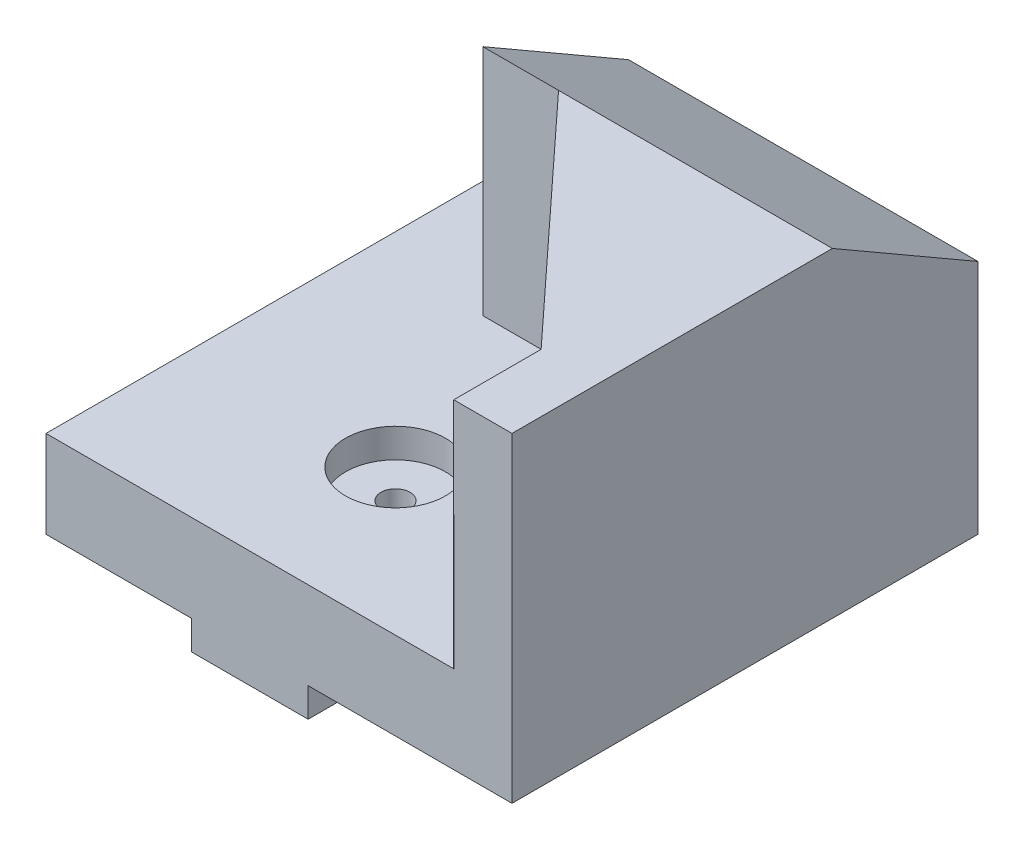
ISO-10303-21;
HEADER;
FILE_DESCRIPTION(('STEP AP214'),'2;1');
FILE_NAME('part.step','',(''),(''),'','','');
FILE_SCHEMA(('AUTOMOTIVE_DESIGN { 1 0 10303 214 1 1 1 1 }'));
ENDSEC;
DATA;
#1=APPLICATION_CONTEXT('core data for automotive mechanical design processes');
#2=APPLICATION_PROTOCOL_DEFINITION('international standard','automotive_design',2000,#1);
#3=PRODUCT_CONTEXT('',#1,'mechanical');
#4=PRODUCT('Part','Part','',(#3));
#5=PRODUCT_RELATED_PRODUCT_CATEGORY('part','',(#4));
#6=PRODUCT_DEFINITION_FORMATION('','',#4);
#7=PRODUCT_DEFINITION_CONTEXT('part definition',#1,'design');
#8=PRODUCT_DEFINITION('design','',#6,#7);
#9=PRODUCT_DEFINITION_SHAPE('','',#8);
#10=(LENGTH_UNIT() NAMED_UNIT(*) SI_UNIT(.MILLI.,.METRE.));
#11=(NAMED_UNIT(*) PLANE_ANGLE_UNIT() SI_UNIT($,.RADIAN.));
#12=(NAMED_UNIT(*) SI_UNIT($,.STERADIAN.) SOLID_ANGLE_UNIT());
#13=UNCERTAINTY_MEASURE_WITH_UNIT(LENGTH_MEASURE(1.E-05),#10,'distance_accuracy_value','');
#14=(GEOMETRIC_REPRESENTATION_CONTEXT(3) GLOBAL_UNCERTAINTY_ASSIGNED_CONTEXT((#13)) GLOBAL_UNIT_ASSIGNED_CONTEXT((#10,
#11,#12)) REPRESENTATION_CONTEXT('',''));
#15=CARTESIAN_POINT('',(0.,0.,0.));
#16=DIRECTION('',(0.,0.,1.));
#17=DIRECTION('',(1.,0.,0.));
#18=AXIS2_PLACEMENT_3D('',#15,#16,#17);
#19=CARTESIAN_POINT('',(-40.,10.,80.));
#20=DIRECTION('',(0.,-1.,0.));
#21=DIRECTION('',(0.,0.,-1.));
#22=AXIS2_PLACEMENT_3D('',#19,#20,#21);
#23=PLANE('',#22);
#24=CARTESIAN_POINT('',(-5.,10.,55.));
#25=DIRECTION('',(0.,1.,0.));
#26=DIRECTION('',(0.,0.,1.));
#27=AXIS2_PLACEMENT_3D('',#24,#25,#26);
#28=CIRCLE('',#27,8.5838793315883);
#29=CARTESIAN_POINT('',(-5.,10.,63.5838793315883));
#30=VERTEX_POINT('',#29);
#31=EDGE_CURVE('E290',#30,#30,#28,.T.);
#32=ORIENTED_EDGE('',*,*,#31,.F.);
#33=EDGE_LOOP('',(#32));
#34=FACE_BOUND('',#33,.T.);
#35=DIRECTION('',(0.679107081248885,0.,0.734039217070601));
#36=VECTOR('',#35,1.);
#37=CARTESIAN_POINT('',(-7.00658305200971,10.,25.));
#38=LINE('',#37,#36);
#39=CARTESIAN_POINT('',(-7.00658305200971,10.,25.));
#40=VERTEX_POINT('',#39);
#41=CARTESIAN_POINT('',(30.,10.,65.));
#42=VERTEX_POINT('',#41);
#43=EDGE_CURVE('E282',#40,#42,#38,.T.);
#44=ORIENTED_EDGE('',*,*,#43,.F.);
#45=DIRECTION('',(1.,0.,0.));
#46=VECTOR('',#45,1.);
#47=CARTESIAN_POINT('',(-7.00658305200971,10.,25.));
#48=LINE('',#47,#46);
#49=CARTESIAN_POINT('',(-20.,10.,25.));
#50=VERTEX_POINT('',#49);
#51=EDGE_CURVE('E278',#50,#40,#48,.T.);
#52=ORIENTED_EDGE('',*,*,#51,.F.);
#53=DIRECTION('',(0.,0.,1.));
#54=VECTOR('',#53,1.);
#55=CARTESIAN_POINT('',(-20.,10.,0.));
#56=LINE('',#55,#54);
#57=CARTESIAN_POINT('',(-20.,10.,0.));
#58=VERTEX_POINT('',#57);
#59=EDGE_CURVE('E149',#58,#50,#56,.T.);
#60=ORIENTED_EDGE('',*,*,#59,.F.);
#61=DIRECTION('',(-1.,0.,0.));
#62=VECTOR('',#61,1.);
#63=CARTESIAN_POINT('',(-40.,10.,0.));
#64=LINE('',#63,#62);
#65=CARTESIAN_POINT('',(-40.,10.,0.));
#66=VERTEX_POINT('',#65);
#67=EDGE_CURVE('E242',#58,#66,#64,.T.);
#68=ORIENTED_EDGE('',*,*,#67,.T.);
#69=DIRECTION('',(0.,0.,-1.));
#70=VECTOR('',#69,1.);
#71=CARTESIAN_POINT('',(-40.,10.,80.));
#72=LINE('',#71,#70);
#73=CARTESIAN_POINT('',(-40.,10.,80.));
#74=VERTEX_POINT('',#73);
#75=EDGE_CURVE('E164',#74,#66,#72,.T.);
#76=ORIENTED_EDGE('',*,*,#75,.F.);
#77=DIRECTION('',(-1.,0.,0.));
#78=VECTOR('',#77,1.);
#79=CARTESIAN_POINT('',(-40.,10.,80.));
#80=LINE('',#79,#78);
#81=CARTESIAN_POINT('',(30.,10.,80.));
#82=VERTEX_POINT('',#81);
#83=EDGE_CURVE('E232',#82,#74,#80,.T.);
#84=ORIENTED_EDGE('',*,*,#83,.F.);
#85=DIRECTION('',(0.,0.,-1.));
#86=VECTOR('',#85,1.);
#87=CARTESIAN_POINT('',(30.,10.,80.));
#88=LINE('',#87,#86);
#89=EDGE_CURVE('E189',#82,#42,#88,.T.);
#90=ORIENTED_EDGE('',*,*,#89,.T.);
#91=EDGE_LOOP('',(#44,#52,#60,#68,#76,#84,#90));
#92=FACE_BOUND('',#91,.T.);
#93=ADVANCED_FACE('F43',(#34,#92),#23,.F.);
#94=CARTESIAN_POINT('',(30.,50.,80.));
#95=DIRECTION('',(-1.,0.,0.));
#96=DIRECTION('',(0.,0.,1.));
#97=AXIS2_PLACEMENT_3D('',#94,#95,#96);
#98=PLANE('',#97);
#99=DIRECTION('',(0.,0.,-1.));
#100=VECTOR('',#99,1.);
#101=CARTESIAN_POINT('',(30.,50.,80.));
#102=LINE('',#101,#100);
#103=CARTESIAN_POINT('',(30.,50.,80.));
#104=VERTEX_POINT('',#103);
#105=CARTESIAN_POINT('',(30.,50.,65.));
#106=VERTEX_POINT('',#105);
#107=EDGE_CURVE('E183',#104,#106,#102,.T.);
#108=ORIENTED_EDGE('',*,*,#107,.T.);
#109=DIRECTION('',(0.,-1.,0.));
#110=VECTOR('',#109,1.);
#111=CARTESIAN_POINT('',(30.,50.,65.));
#112=LINE('',#111,#110);
#113=EDGE_CURVE('E191',#106,#42,#112,.T.);
#114=ORIENTED_EDGE('',*,*,#113,.T.);
#115=ORIENTED_EDGE('',*,*,#89,.F.);
#116=DIRECTION('',(0.,-1.,0.));
#117=VECTOR('',#116,1.);
#118=CARTESIAN_POINT('',(30.,50.,80.));
#119=LINE('',#118,#117);
#120=EDGE_CURVE('E187',#104,#82,#119,.T.);
#121=ORIENTED_EDGE('',*,*,#120,.F.);
#122=EDGE_LOOP('',(#108,#114,#115,#121));
#123=FACE_BOUND('',#122,.T.);
#124=ADVANCED_FACE('F315',(#123),#98,.T.);
#125=CARTESIAN_POINT('',(40.,-10.,80.));
#126=DIRECTION('',(-1.,0.,0.));
#127=DIRECTION('',(0.,0.,1.));
#128=AXIS2_PLACEMENT_3D('',#125,#126,#127);
#129=PLANE('',#128);
#130=DIRECTION('',(0.,1.,0.));
#131=VECTOR('',#130,1.);
#132=CARTESIAN_POINT('',(40.,-10.,0.));
#133=LINE('',#132,#131);
#134=CARTESIAN_POINT('',(40.,-5.,0.));
#135=VERTEX_POINT('',#134);
#136=CARTESIAN_POINT('',(40.,35.5662432702594,0.));
#137=VERTEX_POINT('',#136);
#138=EDGE_CURVE('E214',#135,#137,#133,.T.);
#139=ORIENTED_EDGE('',*,*,#138,.T.);
#140=DIRECTION('',(0.,0.499999999999998,0.86602540378444));
#141=VECTOR('',#140,1.);
#142=CARTESIAN_POINT('',(40.,35.5662432702594,0.));
#143=LINE('',#142,#141);
#144=CARTESIAN_POINT('',(40.,50.,25.0000000000001));
#145=VERTEX_POINT('',#144);
#146=EDGE_CURVE('E58',#137,#145,#143,.T.);
#147=ORIENTED_EDGE('',*,*,#146,.T.);
#148=DIRECTION('',(0.,0.,1.));
#149=VECTOR('',#148,1.);
#150=CARTESIAN_POINT('',(40.,50.,0.));
#151=LINE('',#150,#149);
#152=CARTESIAN_POINT('',(40.,50.,80.));
#153=VERTEX_POINT('',#152);
#154=EDGE_CURVE('E177',#145,#153,#151,.T.);
#155=ORIENTED_EDGE('',*,*,#154,.T.);
#156=DIRECTION('',(0.,1.,0.));
#157=VECTOR('',#156,1.);
#158=CARTESIAN_POINT('',(40.,-10.,80.));
#159=LINE('',#158,#157);
#160=CARTESIAN_POINT('',(40.,-5.,80.));
#161=VERTEX_POINT('',#160);
#162=EDGE_CURVE('E231',#161,#153,#159,.T.);
#163=ORIENTED_EDGE('',*,*,#162,.F.);
#164=DIRECTION('',(0.,0.,1.));
#165=VECTOR('',#164,1.);
#166=CARTESIAN_POINT('',(40.,-5.,0.));
#167=LINE('',#166,#165);
#168=EDGE_CURVE('E220',#135,#161,#167,.T.);
#169=ORIENTED_EDGE('',*,*,#168,.F.);
#170=EDGE_LOOP('',(#139,#147,#155,#163,#169));
#171=FACE_BOUND('',#170,.T.);
#172=ADVANCED_FACE('F318',(#171),#129,.F.);
#173=CARTESIAN_POINT('',(-40.,-10.,80.));
#174=DIRECTION('',(1.,0.,0.));
#175=DIRECTION('',(0.,0.,-1.));
#176=AXIS2_PLACEMENT_3D('',#173,#174,#175);
#177=PLANE('',#176);
#178=DIRECTION('',(0.,0.,1.));
#179=VECTOR('',#178,1.);
#180=CARTESIAN_POINT('',(-40.,-5.,0.));
#181=LINE('',#180,#179);
#182=CARTESIAN_POINT('',(-40.,-5.,0.));
#183=VERTEX_POINT('',#182);
#184=CARTESIAN_POINT('',(-40.,-5.,80.));
#185=VERTEX_POINT('',#184);
#186=EDGE_CURVE('E208',#183,#185,#181,.T.);
#187=ORIENTED_EDGE('',*,*,#186,.T.);
#188=DIRECTION('',(0.,-1.,0.));
#189=VECTOR('',#188,1.);
#190=CARTESIAN_POINT('',(-40.,-10.,80.));
#191=LINE('',#190,#189);
#192=EDGE_CURVE('E238',#74,#185,#191,.T.);
#193=ORIENTED_EDGE('',*,*,#192,.F.);
#194=ORIENTED_EDGE('',*,*,#75,.T.);
#195=DIRECTION('',(0.,-1.,0.));
#196=VECTOR('',#195,1.);
#197=CARTESIAN_POINT('',(-40.,-10.,0.));
#198=LINE('',#197,#196);
#199=EDGE_CURVE('E246',#66,#183,#198,.T.);
#200=ORIENTED_EDGE('',*,*,#199,.T.);
#201=EDGE_LOOP('',(#187,#193,#194,#200));
#202=FACE_BOUND('',#201,.T.);
#203=ADVANCED_FACE('F275',(#202),#177,.F.);
#204=CARTESIAN_POINT('',(-40.,-10.,80.));
#205=DIRECTION('',(0.,1.,0.));
#206=DIRECTION('',(0.,0.,1.));
#207=AXIS2_PLACEMENT_3D('',#204,#205,#206);
#208=PLANE('',#207);
#209=CARTESIAN_POINT('',(-5.,-10.,55.));
#210=DIRECTION('',(0.,1.,0.));
#211=DIRECTION('',(0.,0.,1.));
#212=AXIS2_PLACEMENT_3D('',#209,#210,#211);
#213=CIRCLE('',#212,2.5);
#214=CARTESIAN_POINT('',(-5.,-10.,57.5));
#215=VERTEX_POINT('',#214);
#216=EDGE_CURVE('E48',#215,#215,#213,.T.);
#217=ORIENTED_EDGE('',*,*,#216,.T.);
#218=EDGE_LOOP('',(#217));
#219=FACE_BOUND('',#218,.T.);
#220=DIRECTION('',(0.,0.,1.));
#221=VECTOR('',#220,1.);
#222=CARTESIAN_POINT('',(-15.,-10.,0.));
#223=LINE('',#222,#221);
#224=CARTESIAN_POINT('',(-15.,-10.,0.));
#225=VERTEX_POINT('',#224);
#226=CARTESIAN_POINT('',(-15.,-10.,80.));
#227=VERTEX_POINT('',#226);
#228=EDGE_CURVE('E205',#225,#227,#223,.T.);
#229=ORIENTED_EDGE('',*,*,#228,.F.);
#230=DIRECTION('',(1.,0.,0.));
#231=VECTOR('',#230,1.);
#232=CARTESIAN_POINT('',(-40.,-10.,0.));
#233=LINE('',#232,#231);
#234=CARTESIAN_POINT('',(5.,-10.,0.));
#235=VERTEX_POINT('',#234);
#236=EDGE_CURVE('E236',#225,#235,#233,.T.);
#237=ORIENTED_EDGE('',*,*,#236,.T.);
#238=DIRECTION('',(0.,0.,1.));
#239=VECTOR('',#238,1.);
#240=CARTESIAN_POINT('',(5.,-10.,0.));
#241=LINE('',#240,#239);
#242=CARTESIAN_POINT('',(5.,-10.,80.));
#243=VERTEX_POINT('',#242);
#244=EDGE_CURVE('E196',#235,#243,#241,.T.);
#245=ORIENTED_EDGE('',*,*,#244,.T.);
#246=DIRECTION('',(1.,0.,0.));
#247=VECTOR('',#246,1.);
#248=CARTESIAN_POINT('',(-40.,-10.,80.));
#249=LINE('',#248,#247);
#250=EDGE_CURVE('E169',#227,#243,#249,.T.);
#251=ORIENTED_EDGE('',*,*,#250,.F.);
#252=EDGE_LOOP('',(#229,#237,#245,#251));
#253=FACE_BOUND('',#252,.T.);
#254=ADVANCED_FACE('F255',(#219,#253),#208,.F.);
#255=CARTESIAN_POINT('',(0.,0.,80.));
#256=DIRECTION('',(0.,0.,-1.));
#257=DIRECTION('',(-1.,0.,0.));
#258=AXIS2_PLACEMENT_3D('',#255,#256,#257);
#259=PLANE('',#258);
#260=DIRECTION('',(1.,0.,0.));
#261=VECTOR('',#260,1.);
#262=CARTESIAN_POINT('',(-40.,-5.,80.));
#263=LINE('',#262,#261);
#264=CARTESIAN_POINT('',(-15.,-5.,80.));
#265=VERTEX_POINT('',#264);
#266=EDGE_CURVE('E199',#185,#265,#263,.T.);
#267=ORIENTED_EDGE('',*,*,#266,.T.);
#268=DIRECTION('',(0.,-1.,0.));
#269=VECTOR('',#268,1.);
#270=CARTESIAN_POINT('',(-15.,-5.,80.));
#271=LINE('',#270,#269);
#272=EDGE_CURVE('E201',#265,#227,#271,.T.);
#273=ORIENTED_EDGE('',*,*,#272,.T.);
#274=ORIENTED_EDGE('',*,*,#250,.T.);
#275=DIRECTION('',(0.,1.,0.));
#276=VECTOR('',#275,1.);
#277=CARTESIAN_POINT('',(5.,-10.,80.));
#278=LINE('',#277,#276);
#279=CARTESIAN_POINT('',(5.,-5.,80.));
#280=VERTEX_POINT('',#279);
#281=EDGE_CURVE('E221',#243,#280,#278,.T.);
#282=ORIENTED_EDGE('',*,*,#281,.T.);
#283=DIRECTION('',(1.,0.,0.));
#284=VECTOR('',#283,1.);
#285=CARTESIAN_POINT('',(5.,-5.,80.));
#286=LINE('',#285,#284);
#287=EDGE_CURVE('E210',#280,#161,#286,.T.);
#288=ORIENTED_EDGE('',*,*,#287,.T.);
#289=ORIENTED_EDGE('',*,*,#162,.T.);
#290=DIRECTION('',(1.,0.,0.));
#291=VECTOR('',#290,1.);
#292=CARTESIAN_POINT('',(30.,50.,80.));
#293=LINE('',#292,#291);
#294=EDGE_CURVE('E181',#104,#153,#293,.T.);
#295=ORIENTED_EDGE('',*,*,#294,.F.);
#296=ORIENTED_EDGE('',*,*,#120,.T.);
#297=ORIENTED_EDGE('',*,*,#83,.T.);
#298=ORIENTED_EDGE('',*,*,#192,.T.);
#299=EDGE_LOOP('',(#267,#273,#274,#282,#288,#289,#295,#296,#297,#298));
#300=FACE_BOUND('',#299,.T.);
#301=ADVANCED_FACE('F262',(#300),#259,.F.);
#302=CARTESIAN_POINT('',(0.,0.,0.));
#303=DIRECTION('',(0.,0.,-1.));
#304=DIRECTION('',(-1.,0.,0.));
#305=AXIS2_PLACEMENT_3D('',#302,#303,#304);
#306=PLANE('',#305);
#307=DIRECTION('',(0.,-1.,0.));
#308=VECTOR('',#307,1.);
#309=CARTESIAN_POINT('',(-20.,50.,0.));
#310=LINE('',#309,#308);
#311=CARTESIAN_POINT('',(-20.,35.5662432702594,0.));
#312=VERTEX_POINT('',#311);
#313=EDGE_CURVE('E151',#312,#58,#310,.T.);
#314=ORIENTED_EDGE('',*,*,#313,.F.);
#315=DIRECTION('',(1.,0.,0.));
#316=VECTOR('',#315,1.);
#317=CARTESIAN_POINT('',(40.,35.5662432702594,0.));
#318=LINE('',#317,#316);
#319=EDGE_CURVE('E162',#312,#137,#318,.T.);
#320=ORIENTED_EDGE('',*,*,#319,.T.);
#321=ORIENTED_EDGE('',*,*,#138,.F.);
#322=DIRECTION('',(1.,0.,0.));
#323=VECTOR('',#322,1.);
#324=CARTESIAN_POINT('',(5.,-5.,0.));
#325=LINE('',#324,#323);
#326=CARTESIAN_POINT('',(5.,-5.,0.));
#327=VERTEX_POINT('',#326);
#328=EDGE_CURVE('E227',#327,#135,#325,.T.);
#329=ORIENTED_EDGE('',*,*,#328,.F.);
#330=DIRECTION('',(0.,1.,0.));
#331=VECTOR('',#330,1.);
#332=CARTESIAN_POINT('',(5.,-10.,0.));
#333=LINE('',#332,#331);
#334=EDGE_CURVE('E218',#235,#327,#333,.T.);
#335=ORIENTED_EDGE('',*,*,#334,.F.);
#336=ORIENTED_EDGE('',*,*,#236,.F.);
#337=DIRECTION('',(0.,-1.,0.));
#338=VECTOR('',#337,1.);
#339=CARTESIAN_POINT('',(-15.,-5.,0.));
#340=LINE('',#339,#338);
#341=CARTESIAN_POINT('',(-15.,-5.,0.));
#342=VERTEX_POINT('',#341);
#343=EDGE_CURVE('E200',#342,#225,#340,.T.);
#344=ORIENTED_EDGE('',*,*,#343,.F.);
#345=DIRECTION('',(1.,0.,0.));
#346=VECTOR('',#345,1.);
#347=CARTESIAN_POINT('',(-40.,-5.,0.));
#348=LINE('',#347,#346);
#349=EDGE_CURVE('E198',#183,#342,#348,.T.);
#350=ORIENTED_EDGE('',*,*,#349,.F.);
#351=ORIENTED_EDGE('',*,*,#199,.F.);
#352=ORIENTED_EDGE('',*,*,#67,.F.);
#353=EDGE_LOOP('',(#314,#320,#321,#329,#335,#336,#344,#350,#351,#352));
#354=FACE_BOUND('',#353,.T.);
#355=ADVANCED_FACE('F257',(#354),#306,.T.);
#356=CARTESIAN_POINT('',(5.,-10.,0.));
#357=DIRECTION('',(1.,0.,0.));
#358=DIRECTION('',(0.,0.,-1.));
#359=AXIS2_PLACEMENT_3D('',#356,#357,#358);
#360=PLANE('',#359);
#361=ORIENTED_EDGE('',*,*,#281,.F.);
#362=ORIENTED_EDGE('',*,*,#244,.F.);
#363=ORIENTED_EDGE('',*,*,#334,.T.);
#364=DIRECTION('',(0.,0.,1.));
#365=VECTOR('',#364,1.);
#366=CARTESIAN_POINT('',(5.,-5.,0.));
#367=LINE('',#366,#365);
#368=EDGE_CURVE('E219',#327,#280,#367,.T.);
#369=ORIENTED_EDGE('',*,*,#368,.T.);
#370=EDGE_LOOP('',(#361,#362,#363,#369));
#371=FACE_BOUND('',#370,.T.);
#372=ADVANCED_FACE('F258',(#371),#360,.T.);
#373=CARTESIAN_POINT('',(5.,-5.,0.));
#374=DIRECTION('',(0.,-1.,0.));
#375=DIRECTION('',(0.,0.,-1.));
#376=AXIS2_PLACEMENT_3D('',#373,#374,#375);
#377=PLANE('',#376);
#378=ORIENTED_EDGE('',*,*,#287,.F.);
#379=ORIENTED_EDGE('',*,*,#368,.F.);
#380=ORIENTED_EDGE('',*,*,#328,.T.);
#381=ORIENTED_EDGE('',*,*,#168,.T.);
#382=EDGE_LOOP('',(#378,#379,#380,#381));
#383=FACE_BOUND('',#382,.T.);
#384=ADVANCED_FACE('F335',(#383),#377,.T.);
#385=CARTESIAN_POINT('',(-40.,-5.,0.));
#386=DIRECTION('',(0.,-1.,0.));
#387=DIRECTION('',(0.,0.,-1.));
#388=AXIS2_PLACEMENT_3D('',#385,#386,#387);
#389=PLANE('',#388);
#390=ORIENTED_EDGE('',*,*,#266,.F.);
#391=ORIENTED_EDGE('',*,*,#186,.F.);
#392=ORIENTED_EDGE('',*,*,#349,.T.);
#393=DIRECTION('',(0.,0.,1.));
#394=VECTOR('',#393,1.);
#395=CARTESIAN_POINT('',(-15.,-5.,0.));
#396=LINE('',#395,#394);
#397=EDGE_CURVE('E211',#342,#265,#396,.T.);
#398=ORIENTED_EDGE('',*,*,#397,.T.);
#399=EDGE_LOOP('',(#390,#391,#392,#398));
#400=FACE_BOUND('',#399,.T.);
#401=ADVANCED_FACE('F270',(#400),#389,.T.);
#402=CARTESIAN_POINT('',(-15.,-5.,0.));
#403=DIRECTION('',(-1.,0.,0.));
#404=DIRECTION('',(0.,0.,1.));
#405=AXIS2_PLACEMENT_3D('',#402,#403,#404);
#406=PLANE('',#405);
#407=ORIENTED_EDGE('',*,*,#272,.F.);
#408=ORIENTED_EDGE('',*,*,#397,.F.);
#409=ORIENTED_EDGE('',*,*,#343,.T.);
#410=ORIENTED_EDGE('',*,*,#228,.T.);
#411=EDGE_LOOP('',(#407,#408,#409,#410));
#412=FACE_BOUND('',#411,.T.);
#413=ADVANCED_FACE('F267',(#412),#406,.T.);
#414=CARTESIAN_POINT('',(0.,50.,0.));
#415=DIRECTION('',(0.,-1.,0.));
#416=DIRECTION('',(0.,0.,-1.));
#417=AXIS2_PLACEMENT_3D('',#414,#415,#416);
#418=PLANE('',#417);
#419=ORIENTED_EDGE('',*,*,#154,.F.);
#420=DIRECTION('',(-1.,0.,0.));
#421=VECTOR('',#420,1.);
#422=CARTESIAN_POINT('',(-20.,50.,25.0000000000001));
#423=LINE('',#422,#421);
#424=CARTESIAN_POINT('',(-7.00658305200971,50.,25.));
#425=VERTEX_POINT('',#424);
#426=EDGE_CURVE('E52',#145,#425,#423,.T.);
#427=ORIENTED_EDGE('',*,*,#426,.T.);
#428=DIRECTION('',(0.679107081248885,0.,0.734039217070601));
#429=VECTOR('',#428,1.);
#430=CARTESIAN_POINT('',(-7.00658305200971,50.,25.));
#431=LINE('',#430,#429);
#432=EDGE_CURVE('E158',#425,#106,#431,.T.);
#433=ORIENTED_EDGE('',*,*,#432,.T.);
#434=ORIENTED_EDGE('',*,*,#107,.F.);
#435=ORIENTED_EDGE('',*,*,#294,.T.);
#436=EDGE_LOOP('',(#419,#427,#433,#434,#435));
#437=FACE_BOUND('',#436,.T.);
#438=ADVANCED_FACE('F174',(#437),#418,.F.);
#439=CARTESIAN_POINT('',(-7.00658305200971,50.,25.));
#440=DIRECTION('',(0.734039217070601,0.,-0.679107081248885));
#441=DIRECTION('',(-0.679107081248885,0.,-0.734039217070601));
#442=AXIS2_PLACEMENT_3D('',#439,#440,#441);
#443=PLANE('',#442);
#444=ORIENTED_EDGE('',*,*,#43,.T.);
#445=ORIENTED_EDGE('',*,*,#113,.F.);
#446=ORIENTED_EDGE('',*,*,#432,.F.);
#447=DIRECTION('',(0.,-1.,0.));
#448=VECTOR('',#447,1.);
#449=CARTESIAN_POINT('',(-7.00658305200971,50.,25.));
#450=LINE('',#449,#448);
#451=EDGE_CURVE('E155',#425,#40,#450,.T.);
#452=ORIENTED_EDGE('',*,*,#451,.T.);
#453=EDGE_LOOP('',(#444,#445,#446,#452));
#454=FACE_BOUND('',#453,.T.);
#455=ADVANCED_FACE('F395',(#454),#443,.F.);
#456=CARTESIAN_POINT('',(-20.,50.,0.));
#457=DIRECTION('',(1.,0.,0.));
#458=DIRECTION('',(0.,0.,-1.));
#459=AXIS2_PLACEMENT_3D('',#456,#457,#458);
#460=PLANE('',#459);
#461=DIRECTION('',(0.,-1.,0.));
#462=VECTOR('',#461,1.);
#463=CARTESIAN_POINT('',(-20.,50.,25.));
#464=LINE('',#463,#462);
#465=CARTESIAN_POINT('',(-20.,50.,25.));
#466=VERTEX_POINT('',#465);
#467=EDGE_CURVE('E145',#466,#50,#464,.T.);
#468=ORIENTED_EDGE('',*,*,#467,.F.);
#469=DIRECTION('',(0.,-0.499999999999998,-0.86602540378444));
#470=VECTOR('',#469,1.);
#471=CARTESIAN_POINT('',(-20.,35.5662432702594,0.));
#472=LINE('',#471,#470);
#473=EDGE_CURVE('E11',#466,#312,#472,.T.);
#474=ORIENTED_EDGE('',*,*,#473,.T.);
#475=ORIENTED_EDGE('',*,*,#313,.T.);
#476=ORIENTED_EDGE('',*,*,#59,.T.);
#477=EDGE_LOOP('',(#468,#474,#475,#476));
#478=FACE_BOUND('',#477,.T.);
#479=ADVANCED_FACE('F144',(#478),#460,.F.);
#480=CARTESIAN_POINT('',(-7.00658305200971,50.,25.));
#481=DIRECTION('',(0.,0.,-1.));
#482=DIRECTION('',(-1.,0.,0.));
#483=AXIS2_PLACEMENT_3D('',#480,#481,#482);
#484=PLANE('',#483);
#485=ORIENTED_EDGE('',*,*,#51,.T.);
#486=ORIENTED_EDGE('',*,*,#451,.F.);
#487=DIRECTION('',(1.,0.,0.));
#488=VECTOR('',#487,1.);
#489=CARTESIAN_POINT('',(-7.00658305200971,50.,25.));
#490=LINE('',#489,#488);
#491=EDGE_CURVE('E157',#466,#425,#490,.T.);
#492=ORIENTED_EDGE('',*,*,#491,.F.);
#493=ORIENTED_EDGE('',*,*,#467,.T.);
#494=EDGE_LOOP('',(#485,#486,#492,#493));
#495=FACE_BOUND('',#494,.T.);
#496=ADVANCED_FACE('F159',(#495),#484,.F.);
#497=CARTESIAN_POINT('',(0.,35.5662432702594,0.));
#498=DIRECTION('',(0.,0.86602540378444,-0.499999999999998));
#499=DIRECTION('',(-1.,0.,0.));
#500=AXIS2_PLACEMENT_3D('',#497,#498,#499);
#501=PLANE('',#500);
#502=ORIENTED_EDGE('',*,*,#491,.T.);
#503=ORIENTED_EDGE('',*,*,#426,.F.);
#504=ORIENTED_EDGE('',*,*,#146,.F.);
#505=ORIENTED_EDGE('',*,*,#319,.F.);
#506=ORIENTED_EDGE('',*,*,#473,.F.);
#507=EDGE_LOOP('',(#502,#503,#504,#505,#506));
#508=FACE_BOUND('',#507,.T.);
#509=ADVANCED_FACE('F46',(#508),#501,.T.);
#510=CARTESIAN_POINT('',(-5.,5.,55.));
#511=DIRECTION('',(0.,1.,0.));
#512=DIRECTION('',(0.,0.,1.));
#513=AXIS2_PLACEMENT_3D('',#510,#511,#512);
#514=CYLINDRICAL_SURFACE('',#513,8.5838793315883);
#515=CARTESIAN_POINT('',(-5.,5.,55.));
#516=DIRECTION('',(0.,1.,0.));
#517=DIRECTION('',(0.,0.,1.));
#518=AXIS2_PLACEMENT_3D('',#515,#516,#517);
#519=CIRCLE('',#518,8.5838793315883);
#520=CARTESIAN_POINT('',(-5.,5.,63.5838793315883));
#521=VERTEX_POINT('',#520);
#522=EDGE_CURVE('E284',#521,#521,#519,.T.);
#523=ORIENTED_EDGE('',*,*,#522,.F.);
#524=EDGE_LOOP('',(#523));
#525=FACE_BOUND('',#524,.T.);
#526=ORIENTED_EDGE('',*,*,#31,.T.);
#527=EDGE_LOOP('',(#526));
#528=FACE_BOUND('',#527,.T.);
#529=ADVANCED_FACE('F308',(#525,#528),#514,.F.);
#530=CARTESIAN_POINT('',(-5.,5.,55.));
#531=DIRECTION('',(0.,1.,0.));
#532=DIRECTION('',(0.,0.,1.));
#533=AXIS2_PLACEMENT_3D('',#530,#531,#532);
#534=PLANE('',#533);
#535=CARTESIAN_POINT('',(-5.,5.,55.));
#536=DIRECTION('',(0.,1.,0.));
#537=DIRECTION('',(0.,0.,1.));
#538=AXIS2_PLACEMENT_3D('',#535,#536,#537);
#539=CIRCLE('',#538,2.5);
#540=CARTESIAN_POINT('',(-5.,5.,57.5));
#541=VERTEX_POINT('',#540);
#542=EDGE_CURVE('E291',#541,#541,#539,.T.);
#543=ORIENTED_EDGE('',*,*,#542,.F.);
#544=EDGE_LOOP('',(#543));
#545=FACE_BOUND('',#544,.T.);
#546=ORIENTED_EDGE('',*,*,#522,.T.);
#547=EDGE_LOOP('',(#546));
#548=FACE_BOUND('',#547,.T.);
#549=ADVANCED_FACE('F303',(#545,#548),#534,.T.);
#550=CARTESIAN_POINT('',(-5.,-17.,55.));
#551=DIRECTION('',(0.,1.,0.));
#552=DIRECTION('',(0.,0.,1.));
#553=AXIS2_PLACEMENT_3D('',#550,#551,#552);
#554=CYLINDRICAL_SURFACE('',#553,2.5);
#555=ORIENTED_EDGE('',*,*,#542,.T.);
#556=EDGE_LOOP('',(#555));
#557=FACE_BOUND('',#556,.T.);
#558=ORIENTED_EDGE('',*,*,#216,.F.);
#559=EDGE_LOOP('',(#558));
#560=FACE_BOUND('',#559,.T.);
#561=ADVANCED_FACE('F301',(#557,#560),#554,.F.);
#562=CLOSED_SHELL('',(#93,#124,#172,#203,#254,#301,#355,#372,#384,#401,#413,#438,#455,#479,#496,
#509,#529,#549,#561));
#563=MANIFOLD_SOLID_BREP('B2',#562);
#564=ADVANCED_BREP_SHAPE_REPRESENTATION('',(#18,#563),#14);
#565=SHAPE_DEFINITION_REPRESENTATION(#9,#564);
ENDSEC;
END-ISO-10303-21;
